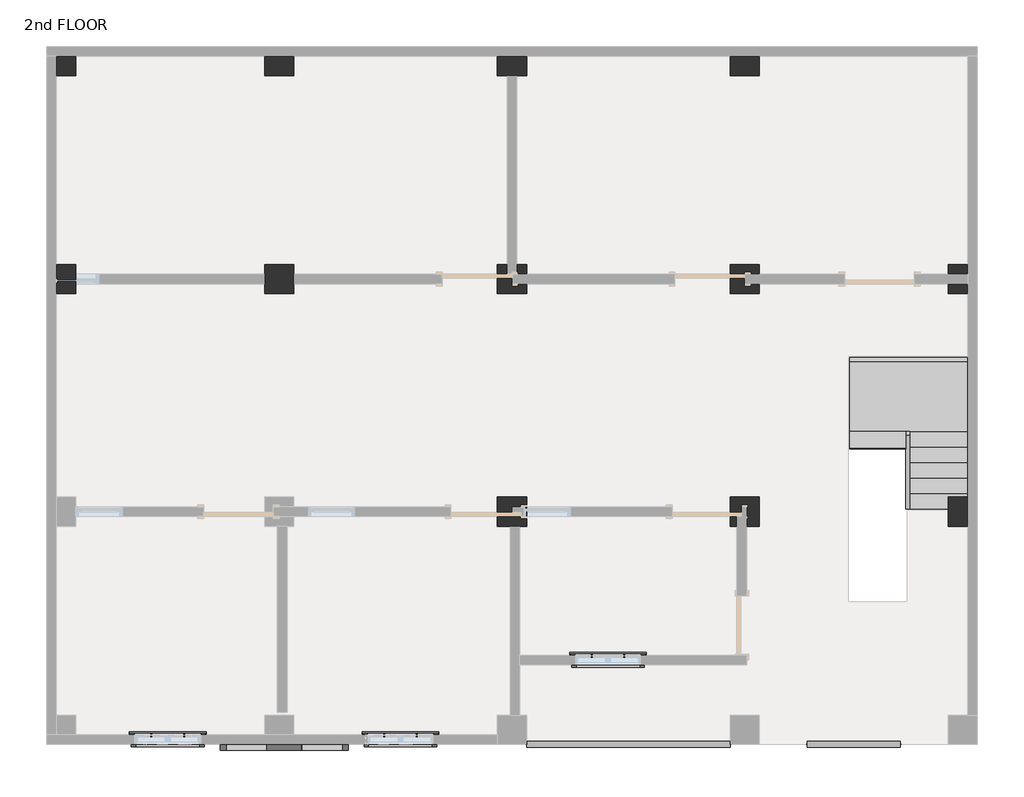
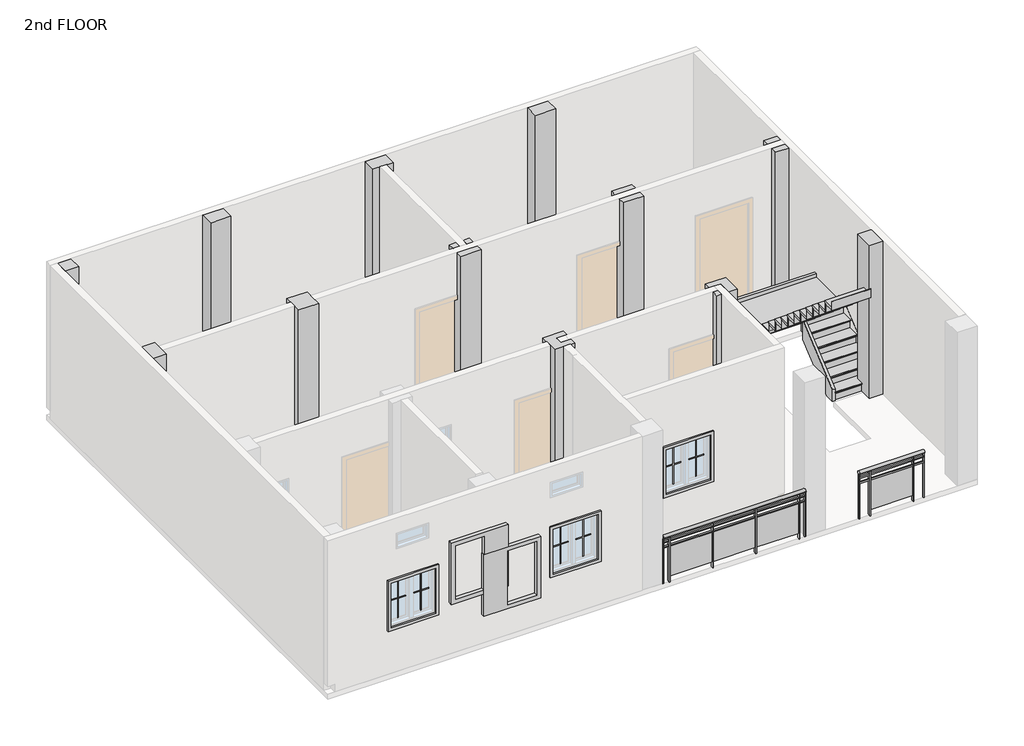
# One storey, part 2 of 2: 12 columns, 12 proxies, 4 members, 2 railings, 1 damper, 1 stair flight.
"""IFC4 building model written with IfcOpenShell, lengths in millimetres."""

from ifc_helpers import new_model, si_unit, point, frame, origin, place, context, project, spatial, polyline, ellipse_curve, trimmed, outline, extrude, faceted_brep, transform, mapped, element, save
from ifc_brep_helpers import plane_surface, extruded_surface, advanced_brep
from components import muntin_pattern_2x2_muntin_pattern_2x2_b3fe6957, muntin_pattern_2x2_muntin_pattern_2x2_3e0ecaf2, trim_window_exterior_flat_with_sill_41619996, trim_window_interior_flat_picture_frame_51c85655, duct_accessories_11_duct_accessories_1_8a8d0748, stair_flight_22957a7c

model = new_model("IFC4")

# Units and contexts
model_context = context("Model", 3, world=origin())
ifc_project = project(units=[si_unit("LENGTHUNIT", "METRE", prefix="MILLI")], contexts=[model_context])

# Site, building, storey
site = spatial("IfcSite", under=ifc_project)
building = spatial("IfcBuilding", under=site)
storey = spatial("IfcBuildingStorey", under=building, Name="2nd FLOOR", Elevation=5943.6)

# Proxies
placement = place(None, origin())
muntin_pattern_2x2_muntin_pattern_2x2_shape = muntin_pattern_2x2_muntin_pattern_2x2_b3fe6957(model_context)
element("IfcBuildingElementProxy", 1, Name="Muntin Pattern_2x2 : Muntin Pattern_2x2", ObjectType="Muntin Pattern_2x2 : Muntin Pattern_2x2", at=placement, inside=storey, context=model_context, shape_type="MappedRepresentation", body=[
    mapped(muntin_pattern_2x2_muntin_pattern_2x2_shape, transform((-14441.409625, -253.8184478, 6927.85), x_axis=(1.0, 0.0, 0.0), y_axis=(0.0, 1.0, 0.0), z_axis=(0.0, 0.0, 1.0))),
])
element("IfcBuildingElementProxy", 2, Name="Muntin Pattern_2x2 : Muntin Pattern_2x2", ObjectType="Muntin Pattern_2x2 : Muntin Pattern_2x2", at=placement, inside=storey, context=model_context, shape_type="MappedRepresentation", body=[
    mapped(muntin_pattern_2x2_muntin_pattern_2x2_shape, transform((-11393.409625, -253.8184478, 6927.85), x_axis=(1.0, 0.0, 0.0), y_axis=(0.0, 1.0, 0.0), z_axis=(0.0, 0.0, 1.0))),
])
element("IfcBuildingElementProxy", 3, Name="Muntin Pattern_2x2 : Muntin Pattern_2x2", ObjectType="Muntin Pattern_2x2 : Muntin Pattern_2x2", at=placement, inside=storey, context=model_context, shape_type="MappedRepresentation", body=[
    mapped(muntin_pattern_2x2_muntin_pattern_2x2_shape, transform((-8675.609625, 787.5815522, 6927.85), x_axis=(1.0, 0.0, 0.0), y_axis=(0.0, 1.0, 0.0), z_axis=(0.0, 0.0, 1.0))),
])
muntin_pattern_2x2_muntin_pattern_2x2_2_shape = muntin_pattern_2x2_muntin_pattern_2x2_3e0ecaf2(model_context)
element("IfcBuildingElementProxy", 4, Name="Muntin Pattern_2x2 : Muntin Pattern_2x2", ObjectType="Muntin Pattern_2x2 : Muntin Pattern_2x2", at=placement, inside=storey, context=model_context, shape_type="MappedRepresentation", body=[
    mapped(muntin_pattern_2x2_muntin_pattern_2x2_2_shape, transform((-14012.784625, -253.8184478, 6927.85), x_axis=(-1.0, 0.0, 0.0), y_axis=(0.0, -1.0, 0.0), z_axis=(0.0, 0.0, 1.0))),
])
element("IfcBuildingElementProxy", 5, Name="Muntin Pattern_2x2 : Muntin Pattern_2x2", ObjectType="Muntin Pattern_2x2 : Muntin Pattern_2x2", at=placement, inside=storey, context=model_context, shape_type="MappedRepresentation", body=[
    mapped(muntin_pattern_2x2_muntin_pattern_2x2_2_shape, transform((-10964.784625, -253.8184478, 6927.85), x_axis=(-1.0, 0.0, 0.0), y_axis=(0.0, -1.0, 0.0), z_axis=(0.0, 0.0, 1.0))),
])
element("IfcBuildingElementProxy", 6, Name="Muntin Pattern_2x2 : Muntin Pattern_2x2", ObjectType="Muntin Pattern_2x2 : Muntin Pattern_2x2", at=placement, inside=storey, context=model_context, shape_type="MappedRepresentation", body=[
    mapped(muntin_pattern_2x2_muntin_pattern_2x2_2_shape, transform((-8246.984625, 787.5815522, 6927.85), x_axis=(-1.0, 0.0, 0.0), y_axis=(0.0, -1.0, 0.0), z_axis=(0.0, 0.0, 1.0))),
])
trim_window_exterior_flat_with_sill_shape = trim_window_exterior_flat_with_sill_41619996(model_context)
element("IfcBuildingElementProxy", 7, Name="Trim-Window-Exterior-Flat : with Sill", ObjectType="Trim-Window-Exterior-Flat : with Sill", at=placement, inside=storey, context=model_context, shape_type="MappedRepresentation", body=[
    mapped(trim_window_exterior_flat_with_sill_shape, transform((-14227.097125, -244.2934478, 7772.4), x_axis=(-1.0, 0.0, 0.0), y_axis=(0.0, 0.0, 1.0), z_axis=(0.0, 1.0, 0.0))),
])
element("IfcBuildingElementProxy", 8, Name="Trim-Window-Exterior-Flat : with Sill", ObjectType="Trim-Window-Exterior-Flat : with Sill", at=placement, inside=storey, context=model_context, shape_type="MappedRepresentation", body=[
    mapped(trim_window_exterior_flat_with_sill_shape, transform((-11179.097125, -244.2934478, 7772.4), x_axis=(-1.0, 0.0, 0.0), y_axis=(0.0, 0.0, 1.0), z_axis=(0.0, 1.0, 0.0))),
])
element("IfcBuildingElementProxy", 9, Name="Trim-Window-Exterior-Flat : with Sill", ObjectType="Trim-Window-Exterior-Flat : with Sill", at=placement, inside=storey, context=model_context, shape_type="MappedRepresentation", body=[
    mapped(trim_window_exterior_flat_with_sill_shape, transform((-8461.297125, 797.1065522, 7772.4), x_axis=(-1.0, 0.0, 0.0), y_axis=(0.0, 0.0, 1.0), z_axis=(0.0, 1.0, 0.0))),
])
trim_window_interior_flat_picture_frame_shape = trim_window_interior_flat_picture_frame_51c85655(model_context)
element("IfcBuildingElementProxy", 10, Name="Trim-Window-Interior-Flat : Picture Frame", ObjectType="Trim-Window-Interior-Flat : Picture Frame", at=placement, inside=storey, context=model_context, shape_type="MappedRepresentation", body=[
    mapped(trim_window_interior_flat_picture_frame_shape, transform((-14227.097125, -371.2934478, 7772.4), x_axis=(1.0, 0.0, 0.0), y_axis=(0.0, 0.0, 1.0), z_axis=(0.0, -1.0, 0.0))),
])
element("IfcBuildingElementProxy", 11, Name="Trim-Window-Interior-Flat : Picture Frame", ObjectType="Trim-Window-Interior-Flat : Picture Frame", at=placement, inside=storey, context=model_context, shape_type="MappedRepresentation", body=[
    mapped(trim_window_interior_flat_picture_frame_shape, transform((-11179.097125, -371.2934478, 7772.4), x_axis=(1.0, 0.0, 0.0), y_axis=(0.0, 0.0, 1.0), z_axis=(0.0, -1.0, 0.0))),
])
element("IfcBuildingElementProxy", 12, Name="Trim-Window-Interior-Flat : Picture Frame", ObjectType="Trim-Window-Interior-Flat : Picture Frame", at=placement, inside=storey, context=model_context, shape_type="MappedRepresentation", body=[
    mapped(trim_window_interior_flat_picture_frame_shape, transform((-8461.297125, 670.1065522, 7772.4), x_axis=(1.0, 0.0, 0.0), y_axis=(0.0, 0.0, 1.0), z_axis=(0.0, -1.0, 0.0))),
])

# Columns
element("IfcColumn", 13, ObjectType="column family : column family", at=placement, inside=storey, context=model_context, shape_type="Brep", body=[
    faceted_brep([(-15433.597125, 8391.7065522, 8986.6), (-15433.597125, 8391.7065522, 5948.6), (-15433.597125, 8645.7065522, 5948.6), (-15433.597125, 8645.7065522, 6096.0), (-15433.597125, 8645.7065522, 8986.6), (-15687.597125, 8391.7065522, 8986.6), (-15687.597125, 8391.7065522, 5948.6), (-15687.597125, 8645.7065522, 8986.6), (-15687.597125, 8645.7065522, 5948.6), (-15687.597125, 8645.7065522, 6096.0)], [[[0, 1, 2, 3, 4]], [[1, 0, 5, 6]], [[0, 4, 7, 5]], [[2, 8, 9, 7, 4, 3]], [[8, 6, 5, 7, 9]], [[2, 1, 6, 8]]]),
])
element("IfcColumn", 14, ObjectType="column family : column family", at=placement, inside=storey, context=model_context, shape_type="SweptSolid", body=[
    extrude(outline(polyline([(-12576.097125, 5915.2065522), (-12576.097125, 5534.2065522), (-12957.097125, 5534.2065522), (-12957.097125, 5915.2065522), (-12576.097125, 5915.2065522)])), frame((0.0, 0.0, 5948.6), z_axis=(0.0, 0.0, 1.0), x_axis=(1.0, 0.0, 0.0)), (0.0, 0.0, 1.0), 3038.0),
])
element("IfcColumn", 15, ObjectType="column family : column family", at=placement, inside=storey, context=model_context, shape_type="Brep", body=[
    faceted_brep([(-9655.097125, 5915.2065522, 5948.6), (-9528.097125, 5915.2065522, 5948.6), (-9528.097125, 5788.2065522, 5948.6), (-9655.097125, 5788.2065522, 5948.6), (-9528.097125, 5915.2065522, 8986.6), (-9655.097125, 5915.2065522, 8986.6), (-9655.097125, 5788.2065522, 8986.6), (-9528.097125, 5788.2065522, 8986.6), (-9655.097125, 5788.2065522, 6096.0), (-9655.097125, 5915.2065522, 6096.0), (-9528.097125, 5788.2065522, 6096.0)], [[[0, 1, 2, 3]], [[4, 5, 6, 7]], [[0, 3, 8, 6, 5, 9]], [[4, 1, 0, 9, 5]], [[3, 2, 10, 7, 6, 8]], [[1, 4, 7, 10, 2]]]),
    faceted_brep([(-9528.097125, 5534.2065522, 8986.6), (-9528.097125, 5534.2065522, 5948.6), (-9528.097125, 5661.2065522, 5948.6), (-9528.097125, 5661.2065522, 6096.0), (-9528.097125, 5661.2065522, 8986.6), (-9909.097125, 5534.2065522, 5948.6), (-9909.097125, 5534.2065522, 8986.6), (-9909.097125, 5661.2065522, 8986.6), (-9909.097125, 5661.2065522, 8077.2), (-9909.097125, 5788.2065522, 8077.2), (-9909.097125, 5788.2065522, 8986.6), (-9909.097125, 5915.2065522, 8986.6), (-9909.097125, 5915.2065522, 5948.6), (-9909.097125, 5788.2065522, 5948.6), (-9909.097125, 5788.2065522, 6096.0), (-9909.097125, 5661.2065522, 6096.0), (-9909.097125, 5661.2065522, 5948.6), (-9782.097125, 5915.2065522, 8986.6), (-9782.097125, 5915.2065522, 6096.0), (-9782.097125, 5915.2065522, 5948.6), (-9782.097125, 5788.2065522, 5948.6), (-9782.097125, 5788.2065522, 8986.6), (-9782.097125, 5788.2065522, 8077.2), (-9782.097125, 5788.2065522, 6096.0), (-9718.597125, 5661.2065522, 5948.6), (-9718.597125, 5661.2065522, 6096.0), (-9718.597125, 5661.2065522, 8077.2), (-9718.597125, 5788.2065522, 8077.2), (-9718.597125, 5788.2065522, 6096.0)], [[[0, 1, 2, 3, 4]], [[5, 1, 0, 6]], [[5, 6, 7, 8, 9, 10, 11, 12, 13, 14, 15, 16]], [[12, 11, 17, 18, 19]], [[20, 19, 18, 17, 21, 22, 23]], [[2, 24, 25, 26, 8, 7, 4, 3]], [[12, 19, 20, 13]], [[6, 0, 4, 7]], [[17, 11, 10, 21]], [[10, 9, 22, 21]], [[27, 26, 25, 28]], [[26, 27, 22, 9, 8]], [[22, 27, 28, 23]], [[15, 25, 24, 16]], [[23, 14, 13, 20]], [[25, 15, 14, 23, 28]], [[1, 5, 16, 24, 2]]]),
])
element("IfcColumn", 16, ObjectType="column family : column family", at=placement, inside=storey, context=model_context, shape_type="Brep", body=[
    faceted_brep([(-6861.097125, 5915.2065522, 5948.6), (-6480.097125, 5915.2065522, 5948.6), (-6480.097125, 5788.2065522, 5948.6), (-6670.597125, 5788.2065522, 5948.6), (-6861.097125, 5788.2065522, 5948.6), (-6480.097125, 5534.2065522, 8986.6), (-6480.097125, 5534.2065522, 5948.6), (-6480.097125, 5661.2065522, 5948.6), (-6480.097125, 5661.2065522, 6096.0), (-6480.097125, 5661.2065522, 8986.6), (-6861.097125, 5534.2065522, 5948.6), (-6861.097125, 5534.2065522, 8986.6), (-6861.097125, 5661.2065522, 8986.6), (-6861.097125, 5661.2065522, 8077.2), (-6861.097125, 5788.2065522, 8077.2), (-6861.097125, 5788.2065522, 8986.6), (-6861.097125, 5915.2065522, 8986.6), (-6861.097125, 5788.2065522, 6096.0), (-6861.097125, 5661.2065522, 6096.0), (-6861.097125, 5661.2065522, 5948.6), (-6480.097125, 5915.2065522, 8986.6), (-6670.597125, 5661.2065522, 5948.6), (-6670.597125, 5661.2065522, 6096.0), (-6670.597125, 5661.2065522, 8077.2), (-6480.097125, 5788.2065522, 6096.0), (-6480.097125, 5788.2065522, 8986.6), (-6670.597125, 5788.2065522, 8077.2), (-6670.597125, 5788.2065522, 6096.0)], [[[0, 1, 2, 3, 4]], [[5, 6, 7, 8, 9]], [[10, 6, 5, 11]], [[10, 11, 12, 13, 14, 15, 16, 0, 4, 17, 18, 19]], [[1, 0, 16, 20]], [[11, 5, 9, 12]], [[7, 21, 22, 23, 13, 12, 9, 8]], [[3, 2, 24, 25, 15, 14, 26, 27]], [[1, 20, 25, 24, 2]], [[20, 16, 15, 25]], [[26, 23, 22, 27]], [[23, 26, 14, 13]], [[18, 22, 21, 19]], [[27, 17, 4, 3]], [[22, 18, 17, 27]], [[6, 10, 19, 21, 7]]]),
])
element("IfcColumn", 17, ObjectType="column family : column family", at=placement, inside=storey, context=model_context, shape_type="Brep", body=[
    faceted_brep([(-6480.097125, 2867.2065522, 5948.6), (-6480.097125, 2486.2065522, 5948.6), (-6645.197125, 2486.2065522, 5948.6), (-6645.197125, 2613.2065522, 5948.6), (-6645.197125, 2740.2065522, 5948.6), (-6708.697125, 2740.2065522, 5948.6), (-6708.697125, 2613.2065522, 5948.6), (-6772.197125, 2613.2065522, 5948.6), (-6772.197125, 2486.2065522, 5948.6), (-6861.097125, 2486.2065522, 5948.6), (-6861.097125, 2867.2065522, 5948.6), (-6480.097125, 2867.2065522, 8986.6), (-6480.097125, 2486.2065522, 8986.6), (-6861.097125, 2486.2065522, 8986.6), (-6772.197125, 2486.2065522, 6096.0), (-6772.197125, 2486.2065522, 8986.6), (-6861.097125, 2613.2065522, 8986.6), (-6861.097125, 2613.2065522, 8077.2), (-6861.097125, 2740.2065522, 8077.2), (-6861.097125, 2740.2065522, 8986.6), (-6861.097125, 2867.2065522, 8986.6), (-6772.197125, 2740.2065522, 8986.6), (-6645.197125, 2740.2065522, 8986.6), (-6645.197125, 2486.2065522, 8986.6), (-6772.197125, 2613.2065522, 8986.6), (-6772.197125, 2613.2065522, 8077.2), (-6772.197125, 2740.2065522, 8077.2), (-6645.197125, 2740.2065522, 6096.0), (-6645.197125, 2613.2065522, 6096.0), (-6645.197125, 2486.2065522, 6096.0), (-6772.197125, 2613.2065522, 6096.0), (-6708.697125, 2613.2065522, 8077.2), (-6708.697125, 2740.2065522, 8077.2), (-6708.697125, 2613.2065522, 6096.0), (-6708.697125, 2740.2065522, 6096.0)], [[[0, 1, 2, 3, 4, 5, 6, 7, 8, 9, 10]], [[1, 0, 11, 12]], [[13, 9, 8, 14, 15]], [[10, 9, 13, 16, 17, 18, 19, 20]], [[0, 10, 20, 11]], [[12, 11, 20, 19, 21, 22, 23]], [[17, 16, 24, 25]], [[19, 18, 26, 21]], [[23, 22, 27, 28, 3, 2, 29]], [[25, 24, 15, 14, 8, 7, 30]], [[16, 13, 15, 24]], [[1, 12, 23, 29, 2]], [[17, 25, 26, 18]], [[25, 31, 32, 26]], [[32, 31, 33, 34]], [[31, 25, 30, 7, 6, 33]], [[26, 32, 34, 27, 22, 21]], [[27, 4, 3, 28]], [[4, 27, 34, 5]], [[5, 34, 33, 6]]]),
])
element("IfcColumn", 18, ObjectType="column family : column family", at=placement, inside=storey, context=model_context, shape_type="Brep", body=[
    faceted_brep([(-9528.097125, 2486.2065522, 5948.6), (-9909.097125, 2486.2065522, 5948.6), (-9909.097125, 2867.2065522, 5948.6), (-9528.097125, 2867.2065522, 5948.6), (-9528.097125, 2740.2065522, 5948.6), (-9566.197125, 2740.2065522, 5948.6), (-9718.597125, 2740.2065522, 5948.6), (-9718.597125, 2613.2065522, 5948.6), (-9566.197125, 2613.2065522, 5948.6), (-9528.097125, 2613.2065522, 5948.6), (-9528.097125, 2486.2065522, 8986.6), (-9528.097125, 2613.2065522, 6096.0), (-9528.097125, 2613.2065522, 6248.4), (-9528.097125, 2740.2065522, 6248.4), (-9528.097125, 2740.2065522, 6096.0), (-9528.097125, 2867.2065522, 8986.6), (-9528.097125, 2740.2065522, 8986.6), (-9528.097125, 2740.2065522, 8077.2), (-9528.097125, 2613.2065522, 8077.2), (-9528.097125, 2613.2065522, 8986.6), (-9909.097125, 2486.2065522, 8986.6), (-9909.097125, 2867.2065522, 8986.6), (-9566.197125, 2613.2065522, 8986.6), (-9718.597125, 2613.2065522, 8986.6), (-9718.597125, 2740.2065522, 8986.6), (-9566.197125, 2740.2065522, 8986.6), (-9718.597125, 2613.2065522, 6096.0), (-9566.197125, 2613.2065522, 8077.2), (-9566.197125, 2613.2065522, 6248.4), (-9566.197125, 2740.2065522, 6248.4), (-9566.197125, 2740.2065522, 8077.2), (-9718.597125, 2740.2065522, 6096.0)], [[[0, 1, 2, 3, 4, 5, 6, 7, 8, 9]], [[10, 0, 9, 11, 12, 13, 14, 4, 3, 15, 16, 17, 18, 19]], [[1, 0, 10, 20]], [[2, 1, 20, 21]], [[3, 2, 21, 15]], [[20, 10, 19, 22, 23, 24, 25, 16, 15, 21]], [[8, 7, 26, 23, 22, 19, 18, 27, 28, 12, 11, 9]], [[5, 4, 14, 13, 29, 30, 17, 16, 25, 24, 31, 6]], [[7, 6, 31, 24, 23, 26]], [[28, 27, 30, 29]], [[28, 29, 13, 12]], [[30, 27, 18, 17]]]),
])
element("IfcColumn", 19, ObjectType="column family : column family", at=placement, inside=storey, context=model_context, shape_type="SweptSolid", body=[
    extrude(outline(polyline([(-12576.097125, 8391.7065522), (-12957.097125, 8391.7065522), (-12957.097125, 8645.7065522), (-12576.097125, 8645.7065522), (-12576.097125, 8391.7065522)])), frame((0.0, 0.0, 5948.6), z_axis=(0.0, 0.0, 1.0), x_axis=(1.0, 0.0, 0.0)), (0.0, 0.0, 1.0), 3038.0),
])
element("IfcColumn", 20, ObjectType="column family : column family", at=placement, inside=storey, context=model_context, shape_type="SweptSolid", body=[
    extrude(outline(polyline([(-9528.097125, 8391.7065522), (-9909.097125, 8391.7065522), (-9909.097125, 8645.7065522), (-9528.097125, 8645.7065522), (-9528.097125, 8391.7065522)])), frame((0.0, 0.0, 5948.6), z_axis=(0.0, 0.0, 1.0), x_axis=(1.0, 0.0, 0.0)), (0.0, 0.0, 1.0), 3038.0),
])
element("IfcColumn", 21, ObjectType="column family : column family", at=placement, inside=storey, context=model_context, shape_type="SweptSolid", body=[
    extrude(outline(polyline([(-6480.097125, 8391.7065522), (-6861.097125, 8391.7065522), (-6861.097125, 8645.7065522), (-6480.097125, 8645.7065522), (-6480.097125, 8391.7065522)])), frame((0.0, 0.0, 5948.6), z_axis=(0.0, 0.0, 1.0), x_axis=(1.0, 0.0, 0.0)), (0.0, 0.0, 1.0), 3038.0),
])
element("IfcColumn", 22, ObjectType="column family : column family", at=placement, inside=storey, context=model_context, shape_type="Brep", body=[
    faceted_brep([(-4003.597125, 5915.2065522, 5948.6), (-3749.597125, 5915.2065522, 5948.6), (-3749.597125, 5788.2065522, 5948.6), (-4003.597125, 5788.2065522, 5948.6), (-4003.597125, 5915.2065522, 8986.6), (-4003.597125, 5788.2065522, 6096.0), (-4003.597125, 5788.2065522, 8986.6), (-3749.597125, 5915.2065522, 8986.6), (-3749.597125, 5788.2065522, 8986.6), (-3749.597125, 5788.2065522, 6096.0)], [[[0, 1, 2, 3]], [[4, 0, 3, 5, 6]], [[0, 4, 7, 1]], [[1, 7, 8, 9, 2]], [[3, 2, 9, 8, 6, 5]], [[7, 4, 6, 8]]]),
    faceted_brep([(-4003.597125, 5534.2065522, 8986.6), (-4003.597125, 5534.2065522, 5948.6), (-3749.597125, 5534.2065522, 5948.6), (-3749.597125, 5534.2065522, 8986.6), (-3749.597125, 5661.2065522, 8986.6), (-4003.597125, 5661.2065522, 8986.6), (-3749.597125, 5661.2065522, 5948.6), (-4003.597125, 5661.2065522, 5948.6), (-4003.597125, 5661.2065522, 6096.0), (-3749.597125, 5661.2065522, 6096.0)], [[[0, 1, 2, 3]], [[0, 3, 4, 5]], [[6, 7, 8, 5, 4, 9]], [[2, 1, 7, 6]], [[3, 2, 6, 9, 4]], [[1, 0, 5, 8, 7]]]),
])
element("IfcColumn", 23, ObjectType="column family : column family", at=placement, inside=storey, context=model_context, shape_type="SweptSolid", body=[
    extrude(outline(polyline([(-4003.597125, 2486.2065522), (-4003.597125, 2867.2065522), (-3749.597125, 2867.2065522), (-3749.597125, 2486.2065522), (-4003.597125, 2486.2065522)])), frame((0.0, 0.0, 5948.6), z_axis=(0.0, 0.0, 1.0), x_axis=(1.0, 0.0, 0.0)), (0.0, 0.0, 1.0), 3038.0),
])
element("IfcColumn", 24, ObjectType="column family : column family", at=placement, inside=storey, context=model_context, shape_type="SweptSolid", body=[
    extrude(outline(polyline([(-15433.597125, 5915.2065522), (-15433.597125, 5534.2065522), (-15687.597125, 5534.2065522), (-15687.597125, 5915.2065522), (-15433.597125, 5915.2065522)])), frame((0.0, 0.0, 5948.6), z_axis=(0.0, 0.0, 1.0), x_axis=(1.0, 0.0, 0.0)), (0.0, 0.0, 1.0), 3038.0),
])

# Damper
duct_accessories_11_duct_accessories_1_shape = duct_accessories_11_duct_accessories_1_8a8d0748(model_context)
element("IfcDamper", 25, ObjectType="Duct Accessories 11 : Duct Accessories 1", at=placement, inside=storey, context=model_context, shape_type="MappedRepresentation", body=[
    mapped(duct_accessories_11_duct_accessories_1_shape, transform((0.0, 0.0, 0.0), x_axis=(1.0, 0.0, 0.0), y_axis=(0.0, 1.0, 0.0), z_axis=(0.0, 0.0, 1.0))),
])

# Members
element("IfcMember", 26, ObjectType="Stringer - 2\" Width", at=placement, inside=storey, context=model_context, shape_type="SweptSolid", body=[
    extrude(outline(polyline([(2714.6319226, 5943.6), (2714.6319226, 6180.4438745), (3679.8319226, 6984.7772078), (3679.8319226, 6588.0165243), (2906.5320935, 5943.6), (2714.6319226, 5943.6)])), frame((-4563.0136682, 0.0, 0.0), z_axis=(1.0, 0.0, 0.0), x_axis=(0.0, 1.0, 0.0)), (0.0, 0.0, 1.0), 50.8),
])
element("IfcMember", 27, ObjectType="Stringer - 2\" Width", at=placement, inside=storey, context=model_context, shape_type="SweptSolid", body=[
    extrude(outline(polyline([(-4512.2136682, 3730.6319226), (-4512.2136682, 3679.8319226), (-4563.0136682, 3679.8319226), (-4563.0136682, 3730.6319226), (-4512.2136682, 3730.6319226)])), frame((0.0, 0.0, 6731.0), z_axis=(0.0, 0.0, 1.0), x_axis=(1.0, 0.0, 0.0)), (0.0, 0.0, 1.0), 304.8),
])
element("IfcMember", 28, ObjectType="Stringer - 2\" Width", at=placement, inside=storey, context=model_context, shape_type="SweptSolid", body=[
    extrude(outline(polyline([(2714.6319226, 5943.6), (2714.6319226, 6180.4438745), (3741.0592732, 7035.8), (4217.1720935, 7035.8), (2906.5320935, 5943.6), (2714.6319226, 5943.6)])), frame((-3749.597125, 0.0, 0.0), z_axis=(1.0, 0.0, 0.0), x_axis=(0.0, 1.0, 0.0)), (0.0, 0.0, 1.0), 50.8),
])
element("IfcMember", 29, ObjectType="Stringer - 2\" Width", at=placement, inside=storey, context=model_context, shape_type="SweptSolid", body=[
    extrude(outline(polyline([(-3698.797125, 4695.8319226), (-3698.797125, 4645.0319226), (-5295.0246464, 4645.0319226), (-5295.0246464, 4695.8319226), (-3698.797125, 4695.8319226)])), frame((0.0, 0.0, 6731.0), z_axis=(0.0, 0.0, 1.0), x_axis=(1.0, 0.0, 0.0)), (0.0, 0.0, 1.0), 304.8),
])

# Railings
element("IfcRailing", 30, ObjectType="Glass Panel - Bottom Fill", at=placement, inside=storey, context=model_context, shape_type="SolidModel", body=[
    advanced_brep(
    [(-9528.097125, -333.1934478, 6858.0), (-9528.097125, -409.3934478, 6858.0), (-6861.097125, -333.1934478, 6858.0), (-6861.097125, -409.3934478, 6858.0)],
    [
        (0, 1, ellipse_curve(frame((-9528.097125, -371.2934478, 6858.0), z_axis=(-1.0, 0.0, 0.0), x_axis=(0.0, -1.0, 0.0)), 38.1, 28.575)),
        (1, 0, ellipse_curve(frame((-9528.097125, -371.2934478, 6858.0), z_axis=(-1.0, 0.0, 0.0), x_axis=(0.0, -1.0, 0.0)), 38.1, 28.575)),
        (2, 3, ellipse_curve(frame((-6861.097125, -371.2934478, 6858.0), z_axis=(1.0, 0.0, 0.0), x_axis=(0.0, -1.0, 0.0)), 38.1, 28.575)),
        (3, 2, ellipse_curve(frame((-6861.097125, -371.2934478, 6858.0), z_axis=(1.0, 0.0, 0.0), x_axis=(0.0, -1.0, 0.0)), 38.1, 28.575)),
        (0, 2),
        (3, 1),
    ],
    [
        plane_surface(frame((-9528.097125, -371.2934478, 6858.0), z_axis=(-1.0, 0.0, 0.0), x_axis=(0.0, 1.0, 0.0))),
        plane_surface(frame((-6861.097125, -371.2934478, 6858.0), z_axis=(1.0, 0.0, 0.0), x_axis=(0.0, 1.0, 0.0))),
        extruded_surface(trimmed(ellipse_curve(frame((-6861.097125, -371.2934478, 6858.0), z_axis=(-1.0, 0.0, 0.0), x_axis=(0.0, -1.0, 0.0)), 38.1, 28.575), [point((-6861.097125, -333.1934478, 6858.0))], [point((-6861.097125, -409.3934478, 6858.0))], True, "CARTESIAN"), (-2667.0, 0.0, 0.0), 2667.0),
        extruded_surface(trimmed(ellipse_curve(frame((-6861.097125, -371.2934478, 6858.0), z_axis=(-1.0, 0.0, 0.0), x_axis=(0.0, -1.0, 0.0)), 38.1, 28.575), [point((-6861.097125, -409.3934478, 6858.0))], [point((-6861.097125, -333.1934478, 6858.0))], True, "CARTESIAN"), (-2667.0, 0.0, 0.0), 2667.0),
    ],
    [
        (0, [[1, 2]]),
        (1, [[3, 4]]),
        (2, [[-1, 5, -4, 6]]),
        (3, [[-2, -6, -3, -5]]),
    ],
),
    extrude(outline(polyline([(-9528.097125, -383.9934478), (-9528.097125, -358.5934478), (-6861.097125, -358.5934478), (-6861.097125, -383.9934478), (-9528.097125, -383.9934478)])), frame((0.0, 0.0, 6743.7), z_axis=(0.0, 0.0, 1.0), x_axis=(1.0, 0.0, 0.0)), (0.0, 0.0, 1.0), 25.4),
    extrude(outline(polyline([(-9528.097125, -383.9934478), (-9528.097125, -358.5934478), (-6861.097125, -358.5934478), (-6861.097125, -383.9934478), (-9528.097125, -383.9934478)])), frame((0.0, 0.0, 6642.1), z_axis=(0.0, 0.0, 1.0), x_axis=(1.0, 0.0, 0.0)), (0.0, 0.0, 1.0), 25.4),
    extrude(outline(polyline([(-6981.747125, -396.6934478), (-6981.747125, -345.8934478), (-6969.047125, -345.8934478), (-6969.047125, -396.6934478), (-6981.747125, -396.6934478)])), frame((0.0, 0.0, 5943.6), z_axis=(0.0, 0.0, 1.0), x_axis=(1.0, 0.0, 0.0)), (0.0, 0.0, 1.0), 885.6788223),
    extrude(outline(polyline([(-7788.197125, -364.7582908), (-6975.397125, -364.7582908), (-6975.397125, -371.1082908), (-7788.197125, -371.1082908), (-7788.197125, -364.7582908)])), frame((0.0, 0.0, 6045.2), z_axis=(0.0, 0.0, 1.0), x_axis=(1.0, 0.0, 0.0)), (0.0, 0.0, 1.0), 596.9),
    extrude(outline(polyline([(-7794.547125, -396.6934478), (-7794.547125, -345.8934478), (-7781.847125, -345.8934478), (-7781.847125, -396.6934478), (-7794.547125, -396.6934478)])), frame((0.0, 0.0, 5943.6), z_axis=(0.0, 0.0, 1.0), x_axis=(1.0, 0.0, 0.0)), (0.0, 0.0, 1.0), 885.6788223),
    extrude(outline(polyline([(-8600.997125, -364.7582908), (-7788.197125, -364.7582908), (-7788.197125, -371.1082908), (-8600.997125, -371.1082908), (-8600.997125, -364.7582908)])), frame((0.0, 0.0, 6045.2), z_axis=(0.0, 0.0, 1.0), x_axis=(1.0, 0.0, 0.0)), (0.0, 0.0, 1.0), 596.9),
    extrude(outline(polyline([(-8607.347125, -396.6934478), (-8607.347125, -345.8934478), (-8594.647125, -345.8934478), (-8594.647125, -396.6934478), (-8607.347125, -396.6934478)])), frame((0.0, 0.0, 5943.6), z_axis=(0.0, 0.0, 1.0), x_axis=(1.0, 0.0, 0.0)), (0.0, 0.0, 1.0), 885.6788223),
    extrude(outline(polyline([(-9413.797125, -364.7582908), (-8600.997125, -364.7582908), (-8600.997125, -371.1082908), (-9413.797125, -371.1082908), (-9413.797125, -364.7582908)])), frame((0.0, 0.0, 6045.2), z_axis=(0.0, 0.0, 1.0), x_axis=(1.0, 0.0, 0.0)), (0.0, 0.0, 1.0), 596.9),
    extrude(outline(polyline([(-9420.147125, -396.6934478), (-9420.147125, -345.8934478), (-9407.447125, -345.8934478), (-9407.447125, -396.6934478), (-9420.147125, -396.6934478)])), frame((0.0, 0.0, 5943.6), z_axis=(0.0, 0.0, 1.0), x_axis=(1.0, 0.0, 0.0)), (0.0, 0.0, 1.0), 885.6788223),
    extrude(outline(polyline([(-6873.797125, -380.8184478), (-6873.797125, -361.7684478), (-6854.747125, -361.7684478), (-6854.747125, -380.8184478), (-6873.797125, -380.8184478)])), frame((0.0, 0.0, 5943.6), z_axis=(0.0, 0.0, 1.0), x_axis=(1.0, 0.0, 0.0)), (0.0, 0.0, 1.0), 885.6788223),
    extrude(outline(polyline([(-9534.447125, -380.8184478), (-9534.447125, -361.7684478), (-9515.397125, -361.7684478), (-9515.397125, -380.8184478), (-9534.447125, -380.8184478)])), frame((0.0, 0.0, 5943.6), z_axis=(0.0, 0.0, 1.0), x_axis=(1.0, 0.0, 0.0)), (0.0, 0.0, 1.0), 885.6788223),
])
element("IfcRailing", 31, ObjectType="Glass Panel - Bottom Fill", at=placement, inside=storey, context=model_context, shape_type="SolidModel", body=[
    advanced_brep(
    [(-5851.447125, -333.1934478, 6858.0), (-5851.447125, -409.3934478, 6858.0), (-4632.247125, -333.1934478, 6858.0), (-4632.247125, -409.3934478, 6858.0)],
    [
        (0, 1, ellipse_curve(frame((-5851.447125, -371.2934478, 6858.0), z_axis=(-1.0, 0.0, 0.0), x_axis=(0.0, -1.0, 0.0)), 38.1, 28.575)),
        (1, 0, ellipse_curve(frame((-5851.447125, -371.2934478, 6858.0), z_axis=(-1.0, 0.0, 0.0), x_axis=(0.0, -1.0, 0.0)), 38.1, 28.575)),
        (2, 3, ellipse_curve(frame((-4632.247125, -371.2934478, 6858.0), z_axis=(1.0, 0.0, 0.0), x_axis=(0.0, -1.0, 0.0)), 38.1, 28.575)),
        (3, 2, ellipse_curve(frame((-4632.247125, -371.2934478, 6858.0), z_axis=(1.0, 0.0, 0.0), x_axis=(0.0, -1.0, 0.0)), 38.1, 28.575)),
        (0, 2),
        (3, 1),
    ],
    [
        plane_surface(frame((-5851.447125, -371.2934478, 6858.0), z_axis=(-1.0, 0.0, 0.0), x_axis=(0.0, 1.0, 0.0))),
        plane_surface(frame((-4632.247125, -371.2934478, 6858.0), z_axis=(1.0, 0.0, 0.0), x_axis=(0.0, 1.0, 0.0))),
        extruded_surface(trimmed(ellipse_curve(frame((-4632.247125, -371.2934478, 6858.0), z_axis=(-1.0, 0.0, 0.0), x_axis=(0.0, -1.0, 0.0)), 38.1, 28.575), [point((-4632.247125, -333.1934478, 6858.0))], [point((-4632.247125, -409.3934478, 6858.0))], True, "CARTESIAN"), (-1219.1999999999998, 0.0, 0.0), 1219.1999999999998),
        extruded_surface(trimmed(ellipse_curve(frame((-4632.247125, -371.2934478, 6858.0), z_axis=(-1.0, 0.0, 0.0), x_axis=(0.0, -1.0, 0.0)), 38.1, 28.575), [point((-4632.247125, -409.3934478, 6858.0))], [point((-4632.247125, -333.1934478, 6858.0))], True, "CARTESIAN"), (-1219.1999999999998, 0.0, 0.0), 1219.1999999999998),
    ],
    [
        (0, [[1, 2]]),
        (1, [[3, 4]]),
        (2, [[-1, 5, -4, 6]]),
        (3, [[-2, -6, -3, -5]]),
    ],
),
    extrude(outline(polyline([(-5851.447125, -383.9934478), (-5851.447125, -358.5934478), (-4632.247125, -358.5934478), (-4632.247125, -383.9934478), (-5851.447125, -383.9934478)])), frame((0.0, 0.0, 6743.7), z_axis=(0.0, 0.0, 1.0), x_axis=(1.0, 0.0, 0.0)), (0.0, 0.0, 1.0), 25.4),
    extrude(outline(polyline([(-5851.447125, -383.9934478), (-5851.447125, -358.5934478), (-4632.247125, -358.5934478), (-4632.247125, -383.9934478), (-5851.447125, -383.9934478)])), frame((0.0, 0.0, 6642.1), z_axis=(0.0, 0.0, 1.0), x_axis=(1.0, 0.0, 0.0)), (0.0, 0.0, 1.0), 25.4),
    extrude(outline(polyline([(-4841.797125, -396.6934478), (-4841.797125, -345.8934478), (-4829.097125, -345.8934478), (-4829.097125, -396.6934478), (-4841.797125, -396.6934478)])), frame((0.0, 0.0, 5943.6), z_axis=(0.0, 0.0, 1.0), x_axis=(1.0, 0.0, 0.0)), (0.0, 0.0, 1.0), 885.6788223),
    extrude(outline(polyline([(-5648.247125, -364.7582908), (-4835.447125, -364.7582908), (-4835.447125, -371.1082908), (-5648.247125, -371.1082908), (-5648.247125, -364.7582908)])), frame((0.0, 0.0, 6045.2), z_axis=(0.0, 0.0, 1.0), x_axis=(1.0, 0.0, 0.0)), (0.0, 0.0, 1.0), 596.9),
    extrude(outline(polyline([(-5654.597125, -396.6934478), (-5654.597125, -345.8934478), (-5641.897125, -345.8934478), (-5641.897125, -396.6934478), (-5654.597125, -396.6934478)])), frame((0.0, 0.0, 5943.6), z_axis=(0.0, 0.0, 1.0), x_axis=(1.0, 0.0, 0.0)), (0.0, 0.0, 1.0), 885.6788223),
    extrude(outline(polyline([(-4644.947125, -380.8184478), (-4644.947125, -361.7684478), (-4625.897125, -361.7684478), (-4625.897125, -380.8184478), (-4644.947125, -380.8184478)])), frame((0.0, 0.0, 5943.6), z_axis=(0.0, 0.0, 1.0), x_axis=(1.0, 0.0, 0.0)), (0.0, 0.0, 1.0), 885.6788223),
    extrude(outline(polyline([(-5857.797125, -380.8184478), (-5857.797125, -361.7684478), (-5838.747125, -361.7684478), (-5838.747125, -380.8184478), (-5857.797125, -380.8184478)])), frame((0.0, 0.0, 5943.6), z_axis=(0.0, 0.0, 1.0), x_axis=(1.0, 0.0, 0.0)), (0.0, 0.0, 1.0), 885.6788223),
])

# Stair flight
stair_flight_shape = stair_flight_22957a7c(model_context)
element("IfcStairFlight", 32, ObjectType="2\" Tread 1\" Nosing 1/4\" Riser", at=placement, inside=storey, context=model_context, shape_type="MappedRepresentation", body=[
    mapped(stair_flight_shape, transform((0.0, 0.0, 0.0), x_axis=(1.0, 0.0, 0.0), y_axis=(0.0, 1.0, 0.0), z_axis=(0.0, 0.0, 1.0))),
])

save(model, "model.ifc")

# Revit data of these elements
# Type "Muntin Pattern_2x2 : Muntin Pattern_2x2"
#   Width [instance default] = 4' - 0"
#   Thickness = 0' - 0 1/2"
#   Height [instance default] = 4' - 0"
#   Distance = 0' - 0 3/4"
#   Interior Material [instance default] = none
#   Exterior Material [instance default] = none
#   Default Elevation = 0
# Type "Trim-Window-Exterior-Flat : with Sill"
#   Trim Width = 0' - 2 1/4"
#   Trim Thickness_Picture Frame = 0' - 1 1/4"
#   Trim Thickness_with Sill = 0' - 0 3/4"
#   Sill Thickness = 0' - 1 1/4"
#   Opening Width [instance default] = 2' - 0"
#   Opening Height [instance default] = 3' - 0"
#   Default Elevation = 4' - 0"
#   Sill = yes
#   Picture Frame = no
#   Trim Material [instance default] = none
# Type "Trim-Window-Interior-Flat : Picture Frame"
#   Trim Thickness_Picture Frame = 0' - 1 1/4"
#   Trim Width = 0' - 2 1/4"
#   Trim Thickness_with Sill = 0' - 0 3/4"
#   Sill Thickness = 0' - 1 1/4"
#   Opening Width [instance default] = 2' - 0"
#   Opening Height [instance default] = 3' - 0"
#   Default Elevation = 4' - 0"
#   Sill = no
#   Picture Frame = yes
#   Trim Material [instance default] = none
# Type "column family : column family"
#   w2 [instance default] = 0' - 9.88189"
#   w1 [instance default] = 0' - 9.01575"
#   Depth = 1' - 11.62205"
#   Width = 1' - 11.62205"
# Type "Glass Panel - Bottom Fill"
#   Assembly Code = "C2010400"
#   built-in parameter 1008612 = 0.0416667 (stored number, unit not read)
#   built-in parameter 1008611 = 0.0416667 (stored number, unit not read)
#   built-in parameter 1008609 = 0.333333 (stored number, unit not read)
#   built-in parameter 1008604 = 0.166667 (stored number, unit not read)
#   built-in parameter 1008603 = 0.166667 (stored number, unit not read)
#   Railing Height = 3' - 0"
#   built-in parameter 1008630 = 2
#   built-in parameter 1008610 = 2
#   built-in parameter 1008618 = Baluster - Square : 3/4"
# Elements 1, 2, 3, 4, 5, 6 (IfcBuildingElementProxy, "Muntin Pattern_2x2 : Muntin Pattern_2x2")
#   Width = 0' - 11 5/8"
#   Height = 2' - 6 1/2"
#   Interior Material = Wood - Stained
#   Exterior Material = Clad - White
#   Phase Created = New Construction
#   Materials on its faces: "Clad - White", "Wood - Stained"
# Elements 7, 8, 9 (IfcBuildingElementProxy, "Trim-Window-Exterior-Flat : with Sill")
#   Opening Width = 2' - 10"
#   Opening Height = 3' - 0"
#   Trim Material = Clad - White
#   Phase Created = New Construction
#   Materials on its faces: "Clad - White"
# Elements 10, 11, 12 (IfcBuildingElementProxy, "Trim-Window-Interior-Flat : Picture Frame")
#   Opening Width = 2' - 10"
#   Opening Height = 3' - 0"
#   Trim Material = Wood - Stained
#   Phase Created = New Construction
#   Materials on its faces: "Wood - Stained"
# Elements 13, 14, 15, 19, 20, 21 (IfcColumn, "column family : column family")
#   w2 = 1' - 3"
#   w1 = 1' - 3"
#   Phase Created = New Construction
#   Materials on its faces: "Default Wall"
# Elements 16, 22, 23 (IfcColumn, "column family : column family")
#   w2 = 1' - 3"
#   w1 = 1' - 3"
#   Phase Created = New Construction
#   Materials on its faces: "grey", "Default Wall"
# Elements 17, 18 (IfcColumn, "column family : column family")
#   w2 = 1' - 3"
#   w1 = 1' - 3"
#   Phase Created = New Construction
#   Materials on its faces: "Default Wall", "inside wall"
# Element 24 (IfcColumn, "column family : column family")
#   w2 = 1' - 3"
#   w1 = 1' - 3"
#   Phase Created = New Construction
#   Materials on its faces: "inside wall", "Default Wall"
# Element 25 (IfcDamper, "Duct Accessories 11 : Duct Accessories 1")
#   Mark = "11"
#   Phase Created = New Construction
#   Materials on its faces: "border"
# Elements 26, 27, 28, 29 (IfcMember, "Stringer - 2\" Width")
#   Phase Created = New Construction
# Elements 30, 31 (IfcRailing, "Glass Panel - Bottom Fill")
#   Phase Created = New Construction
#   Materials on its faces: "Glass"
# Element 32 (IfcStairFlight, "2\" Tread 1\" Nosing 1/4\" Riser")
#   Phase Created = New Construction
# Materials
#   "Clad - White": class "Wood", colour RGB 242 242 238, transparency 0, Cost = 0
#   "Wood - Stained": class "Wood", colour RGB 224 178 126, transparency 0, Cost = 0
#   "Default Wall": colour RGB 128 128 128, transparency 0, Cost = 0
#   "grey": class "Generic", colour RGB 80 80 80, transparency 0, Cost = 0
#   "inside wall": class "Generic", colour RGB 199 224 95, transparency 0, Cost = 0
#   "border": class "Generic", colour RGB 144 144 144, transparency 0, Cost = 0
#   "Glass": class "Glass", colour RGB 0 128 192, transparency 0.75, Description = "Soda Lime Glass", Cost = 0
